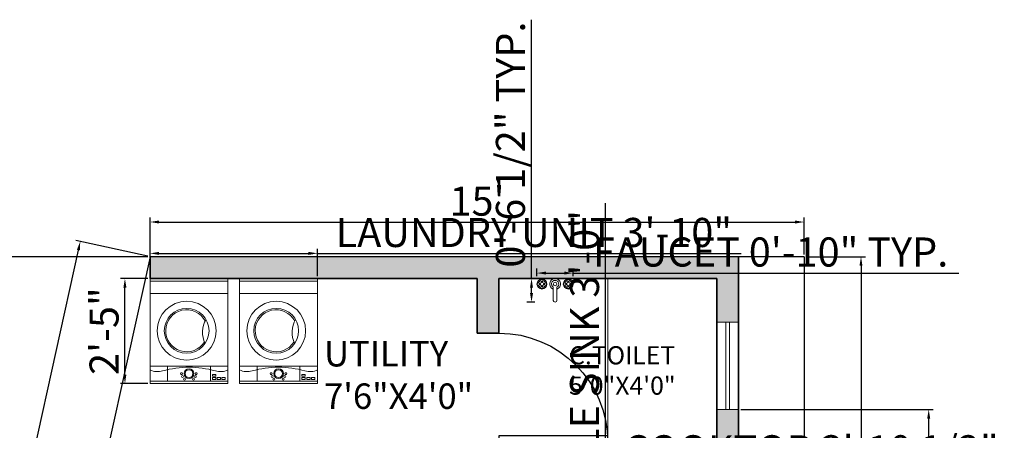
# Model space of a CAD drawing. Units: inches. Extents: x 2642 to 4124, y 1227 to 1973.
# Tile 6 of 7: x 3483 to 3754, y 1860 to 1973. Entities that reach past the tile are written whole.
import ezdxf

# ---------------------------------------------------------------- set-up
doc = ezdxf.new("R2010")
doc.units = ezdxf.units.IN
for name, color, linetype, lineweight in [('A-ANNO-DIMS', 2, 'Continuous', 18), ('A-AREA-IDEN', 7, 'Continuous', 18), ('A-DOOR', 3, 'Continuous', 25), ('A-EQPM', 8, 'Continuous', 18), ('A-WALL', 7, 'Continuous', 35), ('A-WALL-PATT', 7, 'Continuous', 13), ('C-PROP', 7, 'Continuous', 25), ('window', 4, 'Continuous', 18), ('Сантехника', 9, 'Continuous', 18)]:
    doc.layers.add(name, color=color, linetype=linetype, lineweight=lineweight)
doc.styles.get("Standard").update_dxf_attribs({"font": 'arial.ttf'})
doc.dimstyles.new('ISO-25', dxfattribs={"dimtxt": 8, "dimasz": 2.5, "dimexe": 1.25, "dimexo": 0.625, "dimtad": 1, "dimdec": 0, "dimlunit": 3, "dimtxsty": 'Standard', "dimcen": 2.5, "dimadec": 0, "dimazin": 0, "dimtfac": 1, "dimtdec": 0, "dimtmove": 0, "dimatfit": 3, "dimfxl": 1, "dimarcsym": 0})

# ---------------------------------------------------------------- blocks, each defined once
blk = doc.blocks.new('*D1')
at = {"layer": 'A-ANNO-DIMS', "color": 0, "lineweight": -2, "transparency": 16777216}
for p, q in [((3519.22, 1908.41), (3519.22, 1918.57)), ((3521.72, 1917.32), (3696.72, 1917.32)), ((3699.22, 1908.41), (3699.22, 1918.57))]:
    blk.add_line(p, q, dxfattribs=at)
at = {"layer": 'A-ANNO-DIMS', "color": 0, "transparency": 16777216}
for points in [[(3521.72, 1917.74), (3521.72, 1916.9), (3519.22, 1917.32)], [(3696.72, 1917.74), (3696.72, 1916.9), (3699.22, 1917.32)]]:
    blk.add_solid(points, dxfattribs=at)
at = {"layer": 'Defpoints', "color": 0, "transparency": 16777216}
for p in [(3699.22, 1917.32), (3519.22, 1907.78), (3699.22, 1907.78)]:
    blk.add_point(p, dxfattribs=at)
at = {"layer": 'A-ANNO-DIMS', "color": 0, "transparency": 16777216, "insert": (3609.22, 1922.03), "char_height": 8, "attachment_point": 5}
blk.add_mtext("15'", dxfattribs=at)
blk = doc.blocks.new('*D2')
at = {"layer": 'A-ANNO-DIMS', "color": 0, "lineweight": -2, "transparency": 16777216}
for p, q in [((3699.85, 1907.78), (3716.14, 1907.78)), ((3714.89, 1905.28), (3714.89, 1310.28)), ((3699.85, 1307.78), (3716.14, 1307.78))]:
    blk.add_line(p, q, dxfattribs=at)
at = {"layer": 'A-ANNO-DIMS', "color": 0, "transparency": 16777216}
for points in [[(3714.47, 1905.28), (3715.3, 1905.28), (3714.89, 1907.78)], [(3714.47, 1310.28), (3715.3, 1310.28), (3714.89, 1307.78)]]:
    blk.add_solid(points, dxfattribs=at)
at = {"layer": 'Defpoints', "color": 0, "transparency": 16777216}
for p in [(3699.22, 1907.78), (3699.22, 1307.78), (3714.89, 1307.78)]:
    blk.add_point(p, dxfattribs=at)
at = {"layer": 'A-ANNO-DIMS', "color": 0, "transparency": 16777216, "insert": (3710.18, 1607.78), "char_height": 8, "attachment_point": 5, "rotation": 90}
blk.add_mtext("50'", dxfattribs=at)
blk = doc.blocks.new('*D4')
at = {"layer": 'A-ANNO-DIMS', "color": 0, "lineweight": -2, "transparency": 16777216}
for p, q in [((3518.61, 1907.92), (3498.8, 1912.28)), ((3368.56, 1314.45), (3499.49, 1909.57)), ((3386.61, 1307.92), (3366.8, 1312.28))]:
    blk.add_line(p, q, dxfattribs=at)
at = {"layer": 'A-ANNO-DIMS', "color": 0, "transparency": 16777216}
for points in [[(3499.08, 1909.65), (3499.89, 1909.48), (3500.02, 1912.01)], [(3368.15, 1314.54), (3368.97, 1314.36), (3368.02, 1312.01)]]:
    blk.add_solid(points, dxfattribs=at)
at = {"layer": 'Defpoints', "color": 0, "transparency": 16777216}
for p in [(3500.02, 1912.01), (3519.22, 1907.78), (3387.22, 1307.78)]:
    blk.add_point(p, dxfattribs=at)
at = {"layer": 'A-ANNO-DIMS', "color": 0, "transparency": 16777216, "insert": (3429.42, 1613.02), "char_height": 8, "attachment_point": 5, "rotation": 77.5926}
blk.add_mtext('51\'-2"', dxfattribs=at)
blk = doc.blocks.new('*U11')
for p, q in [((0, 0), (0, -6)), ((30, 0), (30, -6))]:
    blk.add_line(p, q)
blk.add_lwpolyline([(0, 0), (0, 30), (1.75, 30), (1.75, 0)], close=True)
blk.add_arc((0, 0), 30, 0, 90)
blk = doc.blocks.new('wash')
at = {"layer": 'Сантехника'}
for p, q in [((4817.13, 2840.92), (4788.24, 2840.92)), ((4788.24, 2819.46), (4788.24, 2840.92)), ((4788.93, 2819.46), (4788.93, 2840.92)), ((4793.08, 2819.46), (4793.08, 2840.92)), ((4812.98, 2819.46), (4812.98, 2840.92)), ((4816.44, 2819.46), (4816.44, 2840.92)), ((4817.13, 2819.46), (4817.13, 2840.92)), ((4793.08, 2836.07), (4788.93, 2836.07)), ((4793.08, 2824.31), (4788.93, 2824.31)), ((4817.13, 2819.46), (4788.24, 2819.46)), ((4817.13, 2816.27), (4788.24, 2816.27)), ((4788.24, 2794.82), (4788.24, 2816.27)), ((4788.93, 2794.82), (4788.93, 2816.27)), ((4793.08, 2794.82), (4793.08, 2816.27)), ((4812.98, 2794.82), (4812.98, 2816.27)), ((4816.44, 2794.82), (4816.44, 2816.27)), ((4817.13, 2794.82), (4817.13, 2816.27)), ((4793.08, 2811.43), (4788.93, 2811.43)), ((4793.08, 2799.66), (4788.93, 2799.66)), ((4817.13, 2794.82), (4788.24, 2794.82))]:
    blk.add_line(p, q, dxfattribs=at)
for points in [[(4789.4, 2839.27), (4789.4, 2840.17), (4789.9, 2840.17), (4789.9, 2839.27)], [(4789.4, 2837.95), (4789.4, 2838.85), (4789.9, 2838.85), (4789.9, 2837.95)], [(4789.4, 2836.64), (4789.4, 2837.53), (4789.9, 2837.53), (4789.9, 2836.64)], [(4790.27, 2836.64), (4790.27, 2837.53), (4790.77, 2837.53), (4790.77, 2836.64)], [(4789.4, 2814.62), (4789.4, 2815.52), (4789.9, 2815.52), (4789.9, 2814.62)], [(4789.4, 2813.31), (4789.4, 2814.2), (4789.9, 2814.2), (4789.9, 2813.31)], [(4789.4, 2811.99), (4789.4, 2812.89), (4789.9, 2812.89), (4789.9, 2811.99)], [(4790.27, 2811.99), (4790.27, 2812.89), (4790.77, 2812.89), (4790.77, 2811.99)]]:
    blk.add_lwpolyline(points, close=True, dxfattribs=at)
for centre, radius in [((4802.77, 2829.54), 8.1), ((4802.77, 2829.54), 6.17), ((4790.19, 2831.93), 0.271), ((4790.98, 2832.18), 0.271), ((4789.46, 2831.45), 0.271), ((4789.46, 2828.92), 0.271), ((4790.98, 2830.19), 1.34), ((4790.98, 2830.19), 1.07), ((4790.19, 2828.4), 0.271), ((4790.98, 2828.15), 0.271), ((4802.77, 2804.9), 8.1), ((4802.77, 2804.9), 6.17), ((4790.19, 2807.28), 0.271), ((4790.98, 2807.53), 0.271), ((4789.46, 2806.8), 0.271), ((4790.98, 2805.55), 1.34), ((4790.98, 2805.55), 1.07), ((4789.46, 2804.27), 0.271), ((4790.19, 2803.75), 0.271), ((4790.98, 2803.5), 0.271)]:
    blk.add_circle(centre, radius, dxfattribs=at)
for centre, radius, start, end in [((4796.44, 2838.85), 4.89, 154.895, 196.6068), ((4762.87, 2829.66), 29.92, 1.0206, 15.0937), ((4802.77, 2829.54), 5.77, 121.8067, 62.1506), ((4802.39, 2840.74), 6.83, 243.19, 300.7673), ((4762.87, 2830.72), 29.92, 344.9063, 358.9794), ((4796.44, 2821.54), 4.89, 163.3932, 205.105), ((4796.44, 2814.2), 4.89, 154.895, 196.6068), ((4762.87, 2805.01), 29.92, 1.0206, 15.0937), ((4802.39, 2816.1), 6.83, 243.19, 300.7673), ((4802.77, 2804.9), 5.77, 121.8067, 62.1506), ((4762.87, 2806.08), 29.92, 344.9063, 358.9794), ((4796.44, 2796.89), 4.89, 163.3932, 205.105)]:
    blk.add_arc(centre, radius, start, end, dxfattribs=at)
blk = doc.blocks.new('Faucet - Bathroom top')
for p, q in [((-4.107, 0.125), (-4.375, 0.125)), ((-3.75, 0.4788), (-3.75, 0.75)), ((-3.5, 0.482), (-3.5, 0.75)), ((-3.1461, 0.125), (-2.875, 0.125)), ((3.143, 0.125), (2.875, 0.125)), ((3.5, 0.4788), (3.5, 0.75)), ((3.75, 0.482), (3.75, 0.75)), ((4.1039, 0.125), (4.375, 0.125)), ((-4.1039, -0.125), (-4.375, -0.125)), ((-3.75, -0.4821), (-3.75, -0.75)), ((-3.5, -0.4789), (-3.5, -0.75)), ((-3.143, -0.125), (-2.875, -0.125)), ((-0.5, -0.8639), (-0.5, -4.5)), ((0.5, -4.5), (0.5, -0.8631)), ((3.1461, -0.125), (2.875, -0.125)), ((3.5, -0.4821), (3.5, -0.75)), ((3.75, -0.4789), (3.75, -0.75)), ((4.107, -0.125), (4.375, -0.125))]:
    blk.add_line(p, q)
for centre, radius in [((-3.625, 0), 1.375), ((-4.625, 0), 0.2795), ((-3.625, 0), 0.5), ((-3.625, 1), 0.2795), ((-2.625, 0), 0.2795), ((0, 0), 0.5), ((3.625, 0), 1.375), ((2.625, 0), 0.2795), ((3.625, 0), 0.5), ((3.625, 1), 0.2795), ((4.625, 0), 0.2795), ((-3.625, -1), 0.2795), ((3.625, -1), 0.2795)]:
    blk.add_circle(centre, radius)
for centre, radius, start, end in [((-3.625, 0), 1, 105.2407, 164.2093), ((-3.625, 0), 1, 16.44125, 74.07887), ((0, 0), 1.5, 289.6514, 250.3603), ((0, 0), 1, 300.3431, 239.7554), ((3.625, 0), 1, 106.12, 164.0884), ((3.625, 0), 1, 16.23422, 73.90469), ((-3.625, 0), 1, 196.2342, 253.9047), ((-3.625, 0), 1, 286.12, 344.0884), ((3.625, 0), 1, 196.4413, 254.0789), ((3.625, 0), 1, 285.2407, 344.2093), ((0, -4.5), 0.5, 180, 0)]:
    blk.add_arc(centre, radius, start, end)
blk = doc.blocks.new('*D46')
at = {"layer": 'A-ANNO-DIMS', "color": 0, "lineweight": -2, "transparency": 16777216}
for p, q in [((3625.71, 1902.41), (3625.71, 1904.53)), ((3628.21, 1903.28), (3633.21, 1903.28)), ((3635.71, 1902.41), (3635.71, 1904.53)), ((3635.71, 1903.28), (3741.79, 1903.28))]:
    blk.add_line(p, q, dxfattribs=at)
at = {"layer": 'A-ANNO-DIMS', "color": 0, "transparency": 16777216}
for points in [[(3628.21, 1903.7), (3628.21, 1902.87), (3625.71, 1903.28)], [(3633.21, 1903.7), (3633.21, 1902.87), (3635.71, 1903.28)]]:
    blk.add_solid(points, dxfattribs=at)
at = {"layer": 'Defpoints', "color": 0, "transparency": 16777216}
for p in [(3635.71, 1903.28), (3625.71, 1901.78), (3635.71, 1901.78)]:
    blk.add_point(p, dxfattribs=at)
at = {"layer": 'A-ANNO-DIMS', "color": 0, "transparency": 16777216, "insert": (3690, 1908.04), "char_height": 8, "attachment_point": 5}
blk.add_mtext('FAUCET 0\'-10" TYP.', dxfattribs=at)
blk = doc.blocks.new('*D47')
at = {"layer": 'A-ANNO-DIMS', "color": 0, "lineweight": -2, "transparency": 16777216}
for p, q in [((3624.21, 1901.78), (3624.21, 1972.94)), ((3625.08, 1901.78), (3622.96, 1901.78)), ((3624.21, 1897.78), (3624.21, 1899.28)), ((3625.08, 1895.28), (3622.96, 1895.28))]:
    blk.add_line(p, q, dxfattribs=at)
at = {"layer": 'A-ANNO-DIMS', "color": 0, "transparency": 16777216}
for points in [[(3623.79, 1899.28), (3624.62, 1899.28), (3624.21, 1901.78)], [(3623.79, 1897.78), (3624.62, 1897.78), (3624.21, 1895.28)]]:
    blk.add_solid(points, dxfattribs=at)
at = {"layer": 'Defpoints', "color": 0, "transparency": 16777216}
for p in [(3624.21, 1901.78), (3625.71, 1901.78), (3625.71, 1895.28)]:
    blk.add_point(p, dxfattribs=at)
at = {"layer": 'A-ANNO-DIMS', "color": 0, "transparency": 16777216, "insert": (3619.44, 1938.61), "char_height": 8, "attachment_point": 5, "rotation": 90}
blk.add_mtext('0\'-6 1/2" TYP.', dxfattribs=at)
blk = doc.blocks.new('*D56')
at = {"layer": 'A-ANNO-DIMS', "color": 0, "lineweight": -2, "transparency": 16777216}
for p, q in [((3519.22, 1902.41), (3519.22, 1909.95)), ((3521.72, 1908.7), (3562.82, 1908.7)), ((3565.32, 1902.41), (3565.32, 1909.95)), ((3565.32, 1908.7), (3681.89, 1908.7))]:
    blk.add_line(p, q, dxfattribs=at)
at = {"layer": 'A-ANNO-DIMS', "color": 0, "transparency": 16777216}
for points in [[(3521.72, 1909.11), (3521.72, 1908.28), (3519.22, 1908.7)], [(3562.82, 1909.11), (3562.82, 1908.28), (3565.32, 1908.7)]]:
    blk.add_solid(points, dxfattribs=at)
at = {"layer": 'Defpoints', "color": 0, "transparency": 16777216}
for p in [(3565.32, 1908.7), (3519.22, 1901.78), (3565.32, 1901.78)]:
    blk.add_point(p, dxfattribs=at)
at = {"layer": 'A-ANNO-DIMS', "color": 0, "transparency": 16777216, "insert": (3624.86, 1913.41), "char_height": 8, "attachment_point": 5}
blk.add_mtext('LAUNDRY UNIT 3\'-10"', dxfattribs=at)
blk = doc.blocks.new('*D57')
at = {"layer": 'A-ANNO-DIMS', "color": 0, "lineweight": -2, "transparency": 16777216}
for p, q in [((3518.6, 1901.78), (3511.06, 1901.78)), ((3512.31, 1875.39), (3512.31, 1899.28)), ((3518.6, 1872.89), (3511.06, 1872.89))]:
    blk.add_line(p, q, dxfattribs=at)
at = {"layer": 'A-ANNO-DIMS', "color": 0, "transparency": 16777216}
for points in [[(3511.89, 1899.28), (3512.72, 1899.28), (3512.31, 1901.78)], [(3511.89, 1875.39), (3512.72, 1875.39), (3512.31, 1872.89)]]:
    blk.add_solid(points, dxfattribs=at)
at = {"layer": 'Defpoints', "color": 0, "transparency": 16777216}
for p in [(3512.31, 1901.78), (3519.22, 1901.78), (3519.22, 1872.89)]:
    blk.add_point(p, dxfattribs=at)
at = {"layer": 'A-ANNO-DIMS', "color": 0, "transparency": 16777216, "insert": (3507.6, 1887.34), "char_height": 8, "attachment_point": 5, "rotation": 90}
blk.add_mtext('2\'-5"', dxfattribs=at)
blk = doc.blocks.new('*D58')
at = {"layer": 'A-ANNO-DIMS', "color": 0, "lineweight": -2, "transparency": 16777216}
for p, q in [((3599.11, 1842.55), (3599.11, 1850.14)), ((3601.61, 1848.89), (3643.06, 1848.89)), ((3645.56, 1842.55), (3645.56, 1850.14)), ((3645.56, 1848.89), (3754.33, 1848.89))]:
    blk.add_line(p, q, dxfattribs=at)
at = {"layer": 'A-ANNO-DIMS', "color": 0, "transparency": 16777216}
for points in [[(3601.61, 1849.31), (3601.61, 1848.48), (3599.11, 1848.89)], [(3643.06, 1849.31), (3643.06, 1848.48), (3645.56, 1848.89)]]:
    blk.add_solid(points, dxfattribs=at)
at = {"layer": 'Defpoints', "color": 0, "transparency": 16777216}
for p in [(3645.56, 1848.89), (3599.11, 1841.93), (3645.56, 1841.93)]:
    blk.add_point(p, dxfattribs=at)
at = {"layer": 'A-ANNO-DIMS', "color": 0, "transparency": 16777216, "insert": (3701.2, 1853.66), "char_height": 8, "attachment_point": 5}
blk.add_mtext('COOKTOP 3\'-10 1/2"', dxfattribs=at)
blk = doc.blocks.new('*D60')
at = {"layer": 'A-ANNO-DIMS', "color": 0, "lineweight": -2, "transparency": 16777216}
for p, q in [((3644.6, 1819.63), (3644.6, 1922.5)), ((3649.37, 1819.63), (3643.35, 1819.63)), ((3644.6, 1786.13), (3644.6, 1817.13)), ((3649.37, 1783.63), (3643.35, 1783.63))]:
    blk.add_line(p, q, dxfattribs=at)
at = {"layer": 'A-ANNO-DIMS', "color": 0, "transparency": 16777216}
for points in [[(3644.18, 1817.13), (3645.02, 1817.13), (3644.6, 1819.63)], [(3644.18, 1786.13), (3645.02, 1786.13), (3644.6, 1783.63)]]:
    blk.add_solid(points, dxfattribs=at)
at = {"layer": 'Defpoints', "color": 0, "transparency": 16777216}
for p in [(3644.6, 1819.63), (3650, 1819.63), (3650, 1783.63)]:
    blk.add_point(p, dxfattribs=at)
at = {"layer": 'A-ANNO-DIMS', "color": 0, "transparency": 16777216, "insert": (3639.83, 1872.32), "char_height": 8, "attachment_point": 5, "rotation": 90}
blk.add_mtext('DOUBLE SINK 3\'-0"', dxfattribs=at)
blk = doc.blocks.new('*D70')
at = {"layer": 'A-ANNO-DIMS', "color": 0, "lineweight": -2, "transparency": 16777216}
for p, q in [((3518.6, 1907.78), (3351.67, 1907.78)), ((3352.92, 1905.28), (3352.92, 1685.28)), ((3485.6, 1682.78), (3351.67, 1682.78))]:
    blk.add_line(p, q, dxfattribs=at)
at = {"layer": 'A-ANNO-DIMS', "color": 0, "transparency": 16777216}
for points in [[(3352.51, 1905.28), (3353.34, 1905.28), (3352.92, 1907.78)], [(3352.51, 1685.28), (3353.34, 1685.28), (3352.92, 1682.78)]]:
    blk.add_solid(points, dxfattribs=at)
at = {"layer": 'Defpoints', "color": 0, "transparency": 16777216}
for p in [(3519.22, 1907.78), (3352.92, 1682.78), (3486.22, 1682.78)]:
    blk.add_point(p, dxfattribs=at)
at = {"layer": 'A-ANNO-DIMS', "color": 0, "transparency": 16777216, "insert": (3348.21, 1795.28), "char_height": 8, "attachment_point": 5, "rotation": 90}
blk.add_mtext('18\'-9"', dxfattribs=at)
blk = doc.blocks.new('*D81')
at = {"layer": 'A-ANNO-DIMS', "color": 0, "lineweight": -2, "transparency": 16777216}
for p, q in [((3681.85, 1865.78), (3734.77, 1865.78)), ((3733.52, 1826.17), (3733.52, 1863.28)), ((3681.85, 1823.67), (3734.77, 1823.67))]:
    blk.add_line(p, q, dxfattribs=at)
at = {"layer": 'A-ANNO-DIMS', "color": 0, "transparency": 16777216}
for points in [[(3733.11, 1863.28), (3733.94, 1863.28), (3733.52, 1865.78)], [(3733.11, 1826.17), (3733.94, 1826.17), (3733.52, 1823.67)]]:
    blk.add_solid(points, dxfattribs=at)
at = {"layer": 'Defpoints', "color": 0, "transparency": 16777216}
for p in [(3681.22, 1865.78), (3733.52, 1865.78), (3681.22, 1823.67)]:
    blk.add_point(p, dxfattribs=at)
at = {"layer": 'A-ANNO-DIMS', "color": 0, "transparency": 16777216, "insert": (3728.81, 1844.73), "char_height": 8, "attachment_point": 5, "rotation": 90}
blk.add_mtext('3\'-6"', dxfattribs=at)

msp = doc.modelspace()

# ---------------------------------------------------------------- hatches: boundary and pattern name
at = {"layer": 'A-WALL-PATT'}
h = msp.add_hatch(color=256, dxfattribs=at)
h.dxf.hatch_style = 1
h.paths.add_polyline_path([(3552.22, 1505.78), (3495.22, 1505.78), (3495.22, 1508.78), (3492.22, 1508.78), (3486.22, 1508.78), (3486.22, 1415.78), (3495.22, 1415.78), (3495.22, 1499.78), (3543.22, 1499.78), (3543.22, 1457.78), (3549.22, 1457.78), (3549.22, 1499.78), (3552.19, 1499.78), (3552.19, 1499.78)])
h.paths.add_polyline_path([(3681.22, 1427.78), (3672.22, 1427.78), (3672.22, 1395.07), (3672.22, 1379.78), (3549.22, 1379.78), (3549.22, 1427.78), (3543.22, 1427.78), (3543.22, 1379.78), (3495.22, 1379.78), (3495.22, 1391.78), (3486.22, 1391.78), (3486.22, 1370.78), (3675.22, 1370.78), (3675.22, 1307.78), (3681.22, 1307.78)])
h.paths.add_polyline_path([(3681.22, 1517.78), (3672.22, 1517.78), (3672.22, 1505.78), (3640.73, 1505.78), (3588.22, 1505.78), (3588.22, 1499.78), (3672.22, 1499.78), (3672.22, 1475.78), (3681.22, 1475.78)])
h.paths.add_polyline_path([(3681.22, 1638.12), (3672.22, 1638.12), (3672.22, 1625.78), (3681.22, 1625.78)])
h.paths.add_polyline_path([(3681.22, 1553.78), (3672.22, 1553.78), (3672.22, 1541.78), (3681.22, 1541.78)])
h.paths.add_polyline_path([(3528.22, 1844.78), (3552.22, 1844.78), (3552.22, 1847.78), (3552.22, 1853.78), (3519.22, 1853.78), (3519.22, 1682.78), (3486.22, 1682.78), (3486.22, 1548.78), (3492.22, 1548.78), (3495.22, 1548.78), (3495.22, 1673.78), (3528.22, 1673.78)])
h.paths.add_polyline_path([(3681.22, 1865.78), (3675.22, 1865.78), (3675.22, 1853.78), (3615.22, 1853.78), (3615.22, 1856.78), (3609.22, 1856.78), (3609.22, 1853.78), (3582.22, 1853.78), (3582.22, 1847.78), (3582.22, 1844.78), (3672.22, 1844.78), (3672.22, 1823.67), (3681.22, 1823.67)])
h.paths.add_polyline_path([(3681.22, 1907.78), (3519.22, 1907.78), (3519.22, 1901.78), (3540.68, 1901.78), (3609.22, 1901.78), (3609.22, 1886.78), (3615.22, 1886.78), (3615.22, 1901.78), (3675.22, 1901.78), (3675.22, 1889.78), (3681.22, 1889.78)])
h.paths.add_polyline_path([(3681.22, 1775.67), (3672.22, 1775.67), (3672.22, 1742.87), (3681.22, 1742.87)])
h.paths.add_polyline_path([(3681.22, 1694.87), (3672.22, 1694.87), (3672.22, 1682.78), (3600.22, 1682.78), (3600.22, 1673.78), (3672.22, 1673.78), (3672.22, 1662.12), (3681.22, 1662.12)])

# ---------------------------------------------------------------- linework, layer by layer
at = {"layer": 'A-WALL'}
for p, q in [((3519.22, 1907.78), (3519.22, 1901.78)), ((3681.22, 1907.78), (3681.22, 1307.78)), ((3609.22, 1901.78), (3519.22, 1901.78)), ((3609.22, 1901.78), (3609.22, 1886.78)), ((3675.22, 1901.78), (3615.22, 1901.78)), ((3615.22, 1901.78), (3615.22, 1886.78)), ((3675.22, 1901.78), (3675.22, 1853.78)), ((3615.22, 1886.78), (3609.22, 1886.78))]:
    msp.add_line(p, q, dxfattribs=at)
at = {"layer": 'C-PROP'}
for p, q in [((3519.22, 1907.78), (3387.22, 1307.78)), ((3699.22, 1907.78), (3519.22, 1907.78)), ((3699.22, 1907.78), (3699.22, 1307.78))]:
    msp.add_line(p, q, dxfattribs=at)
at = {"layer": 'window'}
for p, q in [((3675.22, 1889.78), (3681.22, 1889.78)), ((3677.72, 1889.78), (3677.72, 1865.78)), ((3678.72, 1889.78), (3678.72, 1865.78)), ((3675.22, 1865.78), (3681.22, 1865.78))]:
    msp.add_line(p, q, dxfattribs=at)
at = {"layer": 'Сантехника'}
msp.add_line((3645.21, 1901.48), (3645.21, 1853.48), dxfattribs=at)

# ---------------------------------------------------------------- block references
at = {"layer": 'A-DOOR', "xscale": -1, "rotation": 270}
msp.add_blockref('*U11', (3615.22, 1856.78), dxfattribs=at)
at = {"layer": 'A-EQPM', "xscale": -1, "rotation": 270}
msp.add_blockref('wash', (724.4, -2915.35), dxfattribs=at)
at = {"layer": 'Сантехника'}
msp.add_blockref('Faucet - Bathroom top', (3630.71, 1900.28), dxfattribs=at)

# ---------------------------------------------------------------- texts
at = {"layer": 'A-AREA-IDEN', "attachment_point": 1}
for s, insert, char_height in [('{\\fTimes New Roman|b0|i0|c0|p18;UTILITY\\P7\'6"X4\'0"}', (3567.1, 1884.61), 7), ('{\\fTimes New Roman|b0|i0|c0|p18;C.TOILET\\P5\'0"X4\'0"}', (3634.56, 1883.18), 5)]:
    msp.add_mtext_dynamic_manual_height_columns(s, width=61.0557, gutter_width=12.5, heights=[0], dxfattribs=dict(at, insert=insert, char_height=char_height))

# ---------------------------------------------------------------- dimensions: what is measured, and where the dimension line sits
at = {"layer": 'A-ANNO-DIMS'}
for base, p1, p2, text, picture, middle in [((3624.21, 1901.78), (3625.71, 1895.28), (3625.71, 1901.78), '<> TYP.', '*D47', (3619.44, 1938.61)), ((3644.6, 1819.63), (3650, 1783.63), (3650, 1819.63), 'DOUBLE SINK <>', '*D60', (3639.83, 1872.32))]:
    dim = msp.add_linear_dim(base=base, p1=p1, p2=p2, angle=90, text=text, dimstyle='ISO-25', override={"dimdec": 1, "dimlfac": 1, "dimrnd": 0, "dimzin": 1, "dimdsep": 46, "dimlunit": 4, "dimfrac": 2}, dxfattribs=at)
    dim.commit()
    dim.dimension.update_dxf_attribs({"geometry": picture, "text_midpoint": middle})
for base, p1, p2, text, picture, middle in [((3565.32, 1908.7), (3519.22, 1901.78), (3565.32, 1901.78), 'LAUNDRY UNIT <>', '*D56', (3624.86, 1913.41)), ((3635.71, 1903.28), (3625.71, 1901.78), (3635.71, 1901.78), 'FAUCET <> TYP.', '*D46', (3690, 1908.04)), ((3645.5608, 1848.8932), (3599.1143, 1841.9263), (3645.5608, 1841.9263), 'COOKTOP <>', '*D58', (3701.1961, 1853.6601))]:
    dim = msp.add_linear_dim(base=base, p1=p1, p2=p2, text=text, dimstyle='ISO-25', override={"dimdec": 1, "dimlfac": 1, "dimrnd": 0, "dimzin": 1, "dimdsep": 46, "dimlunit": 4, "dimfrac": 2}, dxfattribs=at)
    dim.commit()
    dim.dimension.update_dxf_attribs({"geometry": picture, "text_midpoint": middle})
dim = msp.add_linear_dim(base=(3699.22, 1917.32), p1=(3519.22, 1907.78), p2=(3699.22, 1907.78), dimstyle='ISO-25', override={"dimclrd": 0, "dimclre": 0, "dimclrt": 0}, dxfattribs=at)
dim.commit()
dim.dimension.update_dxf_attribs({"geometry": '*D1', "text_midpoint": (3609.22, 1922.03)})
dim = msp.add_aligned_dim(p1=(3387.22, 1307.78), p2=(3519.22, 1907.78), distance=19.66, dimstyle='ISO-25', override={"dimclrd": 0, "dimclre": 0, "dimclrt": 0}, dxfattribs=at)
dim.commit()
dim.dimension.update_dxf_attribs({"geometry": '*D4', "text_midpoint": (3429.42, 1613.02)})
for base, p1, p2, override, picture, middle in [((3352.92, 1682.78), (3519.22, 1907.78), (3486.22, 1682.78), {"dimdec": 1, "dimlfac": 1, "dimrnd": 0, "dimzin": 1, "dimdsep": 46, "dimlunit": 4, "dimfrac": 2}, '*D70', (3348.21, 1795.28)), ((3714.89, 1307.78), (3699.22, 1907.78), (3699.22, 1307.78), {"dimclrd": 0, "dimclre": 0, "dimclrt": 0}, '*D2', (3710.18, 1607.78)), ((3512.31, 1901.78), (3519.22, 1872.89), (3519.22, 1901.78), {"dimdec": 1, "dimlfac": 1, "dimrnd": 0, "dimzin": 1, "dimdsep": 46, "dimlunit": 4, "dimfrac": 2}, '*D57', (3507.6, 1887.34)), ((3733.52, 1865.78), (3681.22, 1823.67), (3681.22, 1865.78), {"dimdec": 1, "dimlfac": 1, "dimrnd": 0, "dimzin": 1, "dimdsep": 46, "dimlunit": 4, "dimfrac": 2}, '*D81', (3728.81, 1844.73))]:
    dim = msp.add_linear_dim(base=base, p1=p1, p2=p2, angle=90, dimstyle='ISO-25', override=override, dxfattribs=at)
    dim.commit()
    dim.dimension.update_dxf_attribs({"geometry": picture, "text_midpoint": middle})

doc.saveas('drawing.dxf')
